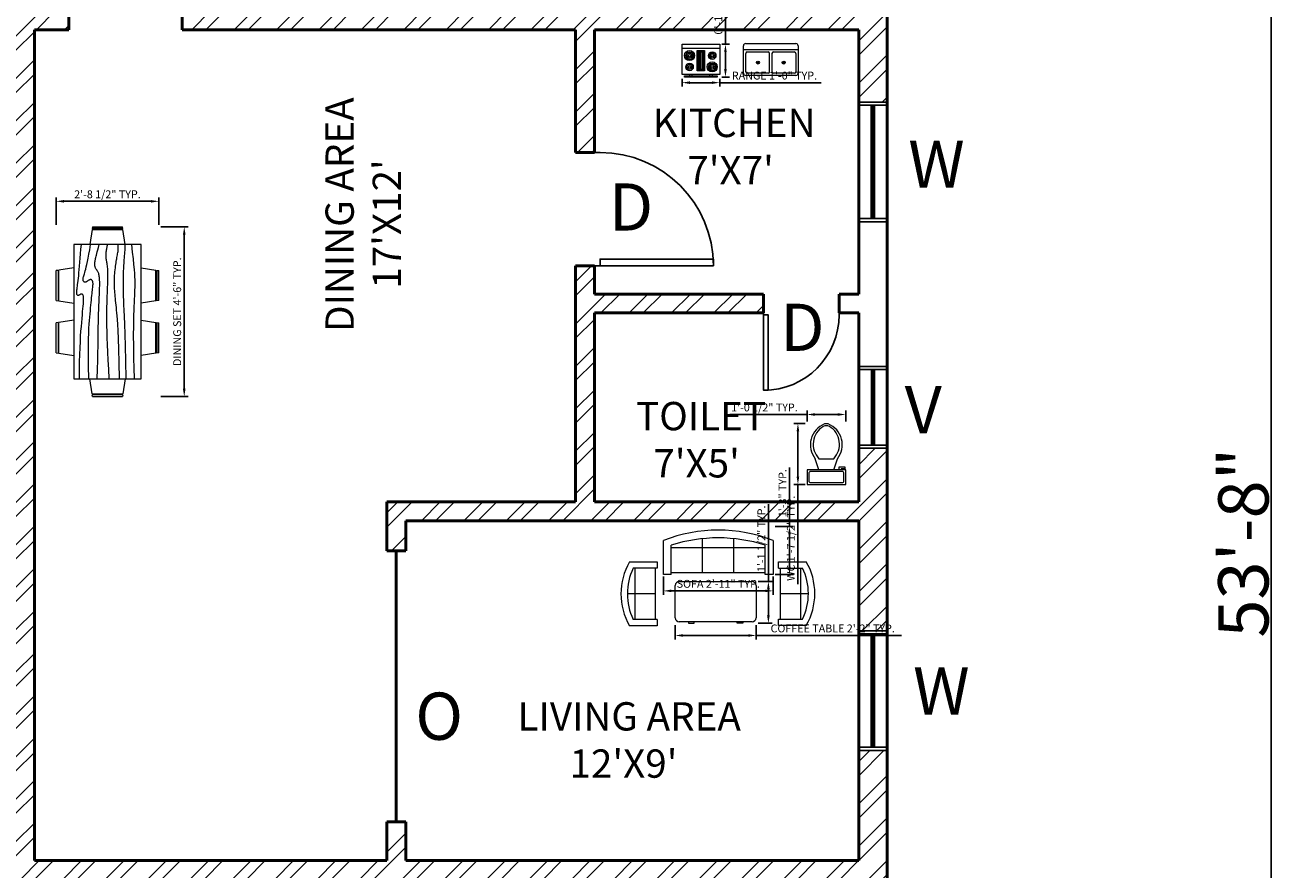
# Model space of a CAD drawing. Units: inches. Extents: x -31485 to -28799, y 18003 to 19130.
# Tile 5 of 15: x -30936 to -30538, y 18398 to 18666. Entities that reach past the tile are written whole.
import ezdxf

# ---------------------------------------------------------------- set-up
doc = ezdxf.new("R2010")
doc.units = ezdxf.units.IN
for name, color, linetype, lineweight in [('A-ANNO-DIMS', 2, 'Continuous', 18), ('A-ANNO-TEXT', 7, 'Continuous', 18), ('A-AREA-IDEN', 7, 'Continuous', 18), ('A-DOOR', 3, 'Continuous', 25), ('A-FLOR-FIXT', 9, 'Continuous', 18), ('A-FURN', 8, 'Continuous', 18), ('A-GLAZ', 4, 'Continuous', 25), ('A-WALL', 7, 'Continuous', 50), ('A-WALL-PATT', 8, 'Continuous', 13)]:
    doc.layers.add(name, color=color, linetype=linetype, lineweight=lineweight)
doc.styles.get("Standard").update_dxf_attribs({"font": 'arial.ttf'})
doc.dimstyles.new('ISO-25', dxfattribs={"dimtxt": 2.5, "dimasz": 2.5, "dimexe": 1.25, "dimexo": 0.625, "dimtad": 1, "dimdec": 0, "dimlunit": 3, "dimtxsty": 'Standard', "dimcen": 2.5, "dimadec": 0, "dimazin": 0, "dimtfac": 1, "dimtdec": 0, "dimtmove": 0, "dimatfit": 3, "dimfxl": 1, "dimarcsym": 0})

# ---------------------------------------------------------------- blocks, each defined once
blk = doc.blocks.new('*U8')
for p, q in [((0, 0), (0, -100)), ((750, 0), (750, -100))]:
    blk.add_line(p, q)
blk.add_lwpolyline([(0, 0), (0, 750), (43.75, 750), (43.75, 0)], close=True)
blk.add_arc((0, 0), 750, 0, 90)
blk = doc.blocks.new('Desk - 30 x 60 in.')
for p, q in [((-26.999995, 0), (26.999995, 0)), ((-29.999995, -27), (-29.999995, -3)), ((29.999995, -3), (29.999995, -27)), ((26.999995, -30), (-26.999995, -30)), ((-20.000005, -30), (-20.000005, -31)), ((-20.000005, -31), (-16.000005, -31)), ((-16.000005, -31), (-16.000005, -30)), ((15.999995, -31), (15.999995, -30)), ((19.999995, -31), (15.999995, -31)), ((19.999995, -30), (19.999995, -31))]:
    blk.add_line(p, q)
for centre, start, end in [((-26.499995, -3.5), 98.1301, 171.8699), ((26.499995, -3.5), 8.130102, 81.8699), ((-26.499995, -26.5), 188.1301, 261.8699), ((26.499995, -26.5), 278.1301, 351.8699)]:
    blk.add_arc(centre, 3.535534, start, end)
blk = doc.blocks.new('Sofa - Roundback 7 ft.')
for p, q in [((-12.00002, -32.4421), (-12.00003, -6.5971)), ((11.99997, -32.4421), (11.99998, -6.5971)), ((-36.000027, -34), (-36.000027, -11.4696)), ((-35.999844, -13.3819), (35.9998, -13.3819)), ((35.99998, -34), (35.99998, -11.4696)), ((-36.000027, -32.4421), (35.99998, -32.4421))]:
    blk.add_line(p, q)
for points in [[(-36.000027, -34), (-42.000027, -34), (-42.000027, -8)], [(41.99998, -8), (41.99998, -34), (35.99998, -34)]]:
    blk.add_lwpolyline(points)
for centre, radius, start, end in [((0, -114.25), 114.25, 68.43141, 111.5686), ((-0.00001, -127.1968), 121.1968, 72.72033, 107.2797)]:
    blk.add_arc(centre, radius, start, end)
blk = doc.blocks.new('Sofa - Roundback Loveseat 5 ft.')
for p, q in [((-24, -33.99998), (-24, -11.46958)), ((0, -32.44198), (0, -5.99998)), ((24.00004, -33.99998), (24.00004, -11.46958)), ((-23.9998, -13.38178), (23.99986, -13.38178)), ((-24, -32.44198), (24.00004, -32.44198))]:
    blk.add_line(p, q)
for points in [[(-24, -33.99998), (-30, -33.99998), (-30, -7.99998)], [(30.00004, -7.99998), (30.00004, -33.99998), (24.00004, -33.99998)]]:
    blk.add_lwpolyline(points)
for centre, radius, start, end in [((0, -60.24998), 60.24998, 60.13715, 119.8628), ((0, -61.38438), 55.38444, 64.32083, 115.6792)]:
    blk.add_arc(centre, radius, start, end)
blk = doc.blocks.new('Dining Set - 36 x 72 in.')
for p, q in [((-22, 27.5), (-22.1562, 26.50042)), ((-22, 27.5), (-6, 27.5)), ((-5.8437, 26.49966), (-6, 27.5)), ((6, 27.5), (5.8438, 26.50042)), ((6, 27.5), (22, 27.5)), ((22.1563, 26.49966), (22, 27.5)), ((-22.2343, 26.00059), (-23.4847, 17.99762)), ((-22.2304, 26), (-5.7608, 26)), ((-5.8416, 26.5), (-22.1534, 26.5)), ((-4.5152, 17.99762), (-5.7655, 25.99926)), ((5.7657, 26.00059), (4.5153, 17.99762)), ((5.7696, 26), (22.2392, 26)), ((22.1584, 26.5), (5.8466, 26.5)), ((23.4848, 17.99762), (22.2345, 25.99926)), ((36, 18), (-36, 18)), ((-36, 18), (-36, -18)), ((36, -18), (36, 18)), ((-45.5, 8), (-44.5004, 8.15617)), ((-45.5, 8), (-45.5, -8)), ((-44.5, -8.15843), (-44.5, 8.15338)), ((-44.0006, 8.23428), (-35.9976, 9.48474)), ((-44, 8.23041), (-44, -8.23915)), ((44.0006, 8.23428), (35.9976, 9.48474)), ((44, 8.23041), (44, -8.23915)), ((44.5, -8.15843), (44.5, 8.15338)), ((45.5, 8), (44.5005, 8.15617)), ((45.5, 8), (45.5, -8)), ((-44.4997, -8.15631), (-45.5, -8)), ((-35.9976, -9.48476), (-43.9993, -8.2345)), ((35.9976, -9.48476), (43.9993, -8.2345)), ((44.4997, -8.15631), (45.5, -8)), ((-36, -18), (36, -18)), ((-22.2343, -26.0006), (-23.4847, -17.99762)), ((-4.5152, -17.99762), (-5.7655, -25.99928)), ((5.7657, -26.0006), (4.5153, -17.99762)), ((23.4848, -17.99762), (22.2345, -25.99928)), ((-22.2304, -26), (-5.7608, -26)), ((-22, -27.5), (-22.1562, -26.50044)), ((-5.8416, -26.5), (-22.1534, -26.5)), ((-5.8437, -26.49967), (-6, -27.5)), ((5.7696, -26), (22.2392, -26)), ((6, -27.5), (5.8438, -26.50044)), ((22.1584, -26.5), (5.8466, -26.5)), ((22.1563, -26.49967), (22, -27.5)), ((-22, -27.5), (-6, -27.5)), ((6, -27.5), (22, -27.5))]:
    blk.add_line(p, q)
for points in [[(-36, 15), (-31.1772, 14.97754), (-26.8079, 14.91406), (-22.8538, 14.81543), (-19.276, 14.6875), (-16.0362, 14.53613), (-13.0957, 14.36718), (-10.4159, 14.18652), (-7.9583, 14), (-5.6904, 13.81315), (-3.6035, 13.63021), (-1.6954, 13.45508), (0.0365, 13.29166), (1.5945, 13.14388), (2.9811, 13.01562), (4.1988, 12.9108), (5.25, 12.83333), (6.1393, 12.78613), (6.8802, 12.76823), (7.4883, 12.77767), (7.9792, 12.8125), (8.3685, 12.87077), (8.6719, 12.95052), (8.9049, 13.0498), (9.0833, 13.16666), (9.2205, 13.29899), (9.3216, 13.44401), (9.3895, 13.59879), (9.4271, 13.76041), (9.4373, 13.92594), (9.4232, 14.09245), (9.3875, 14.257), (9.3333, 14.41666), (9.2638, 14.56917), (9.1836, 14.71484), (9.0975, 14.85465), (9.0104, 14.98958), (8.9272, 15.1206), (8.8529, 15.2487), (8.7922, 15.37483), (8.75, 15.5), (8.7305, 15.62467), (8.7344, 15.74739), (8.7617, 15.86621), (8.8125, 15.97916), (8.8867, 16.08431), (8.9844, 16.17968), (9.1055, 16.26334), (9.25, 16.33333), (9.4189, 16.38802), (9.6172, 16.42708), (9.8506, 16.45052), (10.125, 16.45833), (10.4463, 16.45052), (10.8203, 16.42708), (11.2529, 16.38802), (11.75, 16.33333), (12.3184, 16.26318), (12.9694, 16.17838), (13.7151, 16.07991), (14.5677, 15.96875), (15.5395, 15.84586), (16.6426, 15.71224), (17.8893, 15.56884), (19.2917, 15.41666), (20.859, 15.25667), (22.5879, 15.08984), (24.4721, 14.91715), (26.5052, 14.73958), (28.6809, 14.5581), (30.9929, 14.3737), (33.4347, 14.18733), (36, 14)], [(-36, 10), (-28.9766, 10.14274), (-23.1725, 10.20442), (-18.4241, 10.19775), (-14.5677, 10.13541), (-11.4399, 10.03011), (-8.877, 9.89453), (-6.7154, 9.74137), (-4.7917, 9.58333), (-2.9698, 9.43082), (-1.2246, 9.28515), (0.4415, 9.14534), (2.026, 9.01041), (3.5266, 8.87939), (4.9408, 8.7513), (6.266, 8.62516), (7.5, 8.5), (8.6411, 8.37549), (9.6914, 8.2539), (10.6538, 8.13818), (11.5312, 8.03125), (12.3267, 7.93603), (13.043, 7.85547), (13.6831, 7.79248), (14.25, 7.75), (14.7471, 7.7303), (15.1797, 7.73307), (15.5537, 7.75732), (15.875, 7.80208), (16.1494, 7.86637), (16.3828, 7.94922), (16.5811, 8.04964), (16.75, 8.16666), (16.8944, 8.29915), (17.0143, 8.44531), (17.1089, 8.60319), (17.1771, 8.77083), (17.218, 8.94629), (17.2305, 9.1276), (17.2137, 9.31282), (17.1667, 9.5), (17.0895, 9.6875), (16.987, 9.875), (16.8649, 10.0625), (16.7292, 10.25), (16.5856, 10.4375), (16.4401, 10.625), (16.2985, 10.8125), (16.1667, 11), (16.05, 11.18733), (15.9518, 11.3737), (15.8752, 11.5581), (15.8229, 11.73958), (15.798, 11.91715), (15.8034, 12.08984), (15.842, 12.25667), (15.9167, 12.41666), (16.0295, 12.56836), (16.1784, 12.70833), (16.3605, 12.83268), (16.5729, 12.9375), (16.8127, 13.01888), (17.0768, 13.07291), (17.3625, 13.0957), (17.6667, 13.08333), (17.9894, 13.03312), (18.3418, 12.94726), (18.7382, 12.82918), (19.1927, 12.68229), (19.7195, 12.51001), (20.3327, 12.31575), (21.0465, 12.10294), (21.875, 11.875), (22.8357, 11.63354), (23.959, 11.37304), (25.2786, 11.08618), (26.8282, 10.76562), (28.6414, 10.40405), (30.752, 9.99414), (33.1936, 9.52856), (36, 9)], [(-36, 5.5), (-30.7157, 5.3348), (-26.069, 5.20963), (-21.9946, 5.11767), (-18.4271, 5.05208), (-15.3009, 5.00602), (-12.5508, 4.97265), (-10.1112, 4.94515), (-7.9167, 4.91666), (-5.909, 4.88167), (-4.0586, 4.83984), (-2.3429, 4.79215), (-0.7396, 4.73958), (0.7739, 4.6831), (2.22, 4.6237), (3.6213, 4.56233), (5, 4.5), (6.373, 4.43782), (7.7344, 4.3776), (9.0723, 4.32129), (10.375, 4.27083), (11.6309, 4.22819), (12.8281, 4.19531), (13.9551, 4.17415), (15, 4.16666), (15.954, 4.17448), (16.819, 4.19791), (17.6001, 4.23698), (18.3021, 4.29166), (18.9299, 4.36198), (19.4883, 4.44791), (19.9823, 4.54948), (20.4167, 4.66666), (20.7969, 4.79899), (21.1302, 4.94401), (21.4245, 5.09879), (21.6875, 5.26041), (21.9271, 5.42594), (22.1511, 5.59245), (22.3672, 5.757), (22.5834, 5.91666), (22.8065, 6.06868), (23.0404, 6.21093), (23.2879, 6.34147), (23.5521, 6.45833), (23.8358, 6.55957), (24.142, 6.64323), (24.4735, 6.70735), (24.8334, 6.75), (25.2235, 6.76969), (25.642, 6.76692), (26.0858, 6.74267), (26.5521, 6.69791), (27.0379, 6.63362), (27.5404, 6.55078), (28.0565, 6.45036), (28.5834, 6.33333), (29.1242, 6.19987), (29.7071, 6.04687), (30.3661, 5.87044), (31.1354, 5.66666), (32.0493, 5.43164), (33.142, 5.16146), (34.4475, 4.85221), (36, 4.5)], [(-36, -1), (-30.7915, -0.6591), (-26.0195, -0.38216), (-21.6519, -0.16284), (-17.6563, 0.00521), (-14.0005, 0.12833), (-10.6523, 0.21289), (-7.5796, 0.26522), (-4.75, 0.29166), (-2.134, 0.29793), (0.2878, 0.28711), (2.5317, 0.26163), (4.6146, 0.22396), (6.5529, 0.17651), (8.3633, 0.12174), (10.0623, 0.06209), (11.6667, 0), (13.1899, -0.06201), (14.6341, -0.1211), (15.9982, -0.17432), (17.2813, -0.21875), (18.4823, -0.25147), (19.6003, -0.26953), (20.6343, -0.27002), (21.5834, -0.25), (22.4481, -0.20768), (23.2357, -0.14584), (23.9549, -0.06836), (24.6146, 0.02083), (25.2235, 0.11784), (25.7904, 0.21875), (26.3241, 0.31966), (26.8334, 0.41666), (27.3265, 0.50618), (27.8099, 0.58593), (28.2894, 0.65397), (28.7709, 0.70833), (29.2601, 0.74707), (29.763, 0.76823), (30.2855, 0.76985), (30.8334, 0.75), (31.4088, 0.70784), (31.9994, 0.64713), (32.589, 0.57275), (33.1615, 0.48958), (33.7008, 0.4025), (34.1908, 0.3164), (34.6153, 0.23616), (34.9584, 0.16666), (35.2099, 0.11165), (35.3848, 0.07031), (35.504, 0.04069), (35.5886, 0.02083), (35.6594, 0.00879), (35.7377, 0.0026), (35.8442, 0.00032), (36, 0)], [(-36, -6.5), (-27.1843, -6.31267), (-20.084, -6.1263), (-14.469, -5.9419), (-10.1094, -5.76042), (-6.7752, -5.58285), (-4.2363, -5.41016), (-2.2629, -5.24333), (-0.625, -5.08334), (0.8708, -4.93099), (2.2715, -4.78646), (3.5872, -4.64974), (4.8281, -4.52084), (6.0046, -4.39974), (7.127, -4.28646), (8.2053, -4.18099), (9.25, -4.08334), (10.2705, -3.99382), (11.2734, -3.91407), (12.2647, -3.84603), (13.25, -3.79167), (14.2354, -3.75293), (15.2266, -3.73177), (16.2295, -3.73015), (17.25, -3.75), (18.2912, -3.79248), (19.3451, -3.85547), (20.4009, -3.93604), (21.4479, -4.03125), (22.4754, -4.13819), (23.4727, -4.25391), (24.4289, -4.37549), (25.3334, -4.5), (26.1785, -4.62492), (26.9694, -4.74935), (27.7145, -4.87281), (28.4219, -4.99479), (29.1, -5.11483), (29.7572, -5.23242), (30.4016, -5.34709), (31.0417, -5.45834), (31.6837, -5.56437), (32.3262, -5.65821), (32.9658, -5.73153), (33.599, -5.77604), (34.2224, -5.78345), (34.8327, -5.74545), (35.4264, -5.65373), (36, -5.5)], [(-36, -10), (-26.4022, -9.81299), (-18.4675, -9.62891), (-11.9839, -9.45069), (-6.7396, -9.28125), (-2.5226, -9.12354), (0.8789, -8.98047), (3.6769, -8.85498), (6.0833, -8.75), (8.2767, -8.66765), (10.3021, -8.60677), (12.1712, -8.56543), (13.8958, -8.54167), (15.4876, -8.53353), (16.9583, -8.53907), (18.3197, -8.55632), (19.5834, -8.58334), (20.7616, -8.61841), (21.8685, -8.66081), (22.9188, -8.71004), (23.9271, -8.76563), (24.9081, -8.82707), (25.8763, -8.89388), (26.8465, -8.96558), (27.8334, -9.04167), (28.8474, -9.12118), (29.8828, -9.20117), (30.93, -9.27824), (31.9792, -9.34896), (33.0205, -9.40991), (34.0443, -9.45768), (35.0407, -9.48885), (36, -9.5)], [(-36, -14.5), (-30.0881, -14.33513), (-25.0332, -14.21224), (-20.7312, -14.12647), (-17.0781, -14.07292), (-13.97, -14.04671), (-11.3027, -14.04297), (-8.9724, -14.05681), (-6.875, -14.08334), (-4.9224, -14.11833), (-3.0905, -14.16016), (-1.3709, -14.20785), (0.2448, -14.26042), (1.7647, -14.3169), (3.1973, -14.3763), (4.5507, -14.43767), (5.8333, -14.5), (7.0554, -14.5621), (8.235, -14.62175), (9.3922, -14.67652), (10.5469, -14.72396), (11.7192, -14.76164), (12.929, -14.78711), (14.1965, -14.79794), (15.5417, -14.79167), (16.9933, -14.76424), (18.6152, -14.70508), (20.4804, -14.60197), (22.6615, -14.44271), (25.2312, -14.21509), (28.2624, -13.9069), (31.8277, -13.50594), (36, -13)]]:
    blk.add_lwpolyline(points)
blk = doc.blocks.new('Range-Oven - 30 in top')
for p, q in [((0, -3), (30, -3)), ((12, -6), (18, -6)), ((13, -20), (13, -6)), ((14, -6), (14, -20)), ((15, -20), (15, -6)), ((16, -6), (16, -20)), ((17, -20), (17, -6)), ((6, -24), (6, -25)), ((8, -25), (8, -24)), ((18, -20), (12, -20)), ((22, -25), (22, -24)), ((24, -24), (24, -25))]:
    blk.add_line(p, q)
for points in [[(0, -24), (0, 0), (30, 0), (30, -24)], [(12, -21), (12, -5), (18, -5), (18, -21)], [(2, -26), (2, -25), (28, -25), (28, -26)]]:
    blk.add_lwpolyline(points, close=True)
for centre, radius in [((6, -9), 4), ((6, -9), 3), ((6, -9), 2), ((6, -9), 1), ((24, -9), 3), ((24, -9), 2), ((24, -9), 1), ((6, -18), 3), ((6, -18), 2), ((6, -18), 1), ((24, -18), 4), ((24, -18), 3), ((24, -18), 2), ((24, -18), 1)]:
    blk.add_circle(centre, radius)
blk = doc.blocks.new('Sink-double - 36 in top')
for p, q in [((-18, -4), (18, -4)), ((-0.75, -18.5), (-0.75, -6.5)), ((0.75, -6.5), (0.75, -18.5))]:
    blk.add_line(p, q)
for points in [[(-16.5, 0), (16.5, 0)], [(-18, -19.5), (-18, -1.5)], [(-16.5, -18.5), (-16.5, -6.5)], [(-15.5, -5.5), (-1.75, -5.5)], [(1.75, -5.5), (15.5, -5.5)], [(16.5, -6.5), (16.5, -18.5)], [(18, -1.5), (18, -19.5)], [(16.5, -21), (-16.5, -21)], [(-1.75, -19.5), (-15.5, -19.5)], [(15.5, -19.5), (1.75, -19.5)]]:
    blk.add_lwpolyline(points)
for centre, radius in [((-8.5, -12.5), 1), ((-8.5, -12.5), 0.5), ((8.5, -12.5), 1), ((8.5, -12.5), 0.5)]:
    blk.add_circle(centre, radius)
for centre, radius, start, end in [((-16.5, -1.5), 1.5, 90, 180), ((16.5, -1.5), 1.5, 0, 90), ((-15.5, -6.5), 1, 90, 180), ((-1.75, -6.5), 1, 0, 90), ((1.75, -6.5), 1, 90, 180), ((15.5, -6.5), 1, 0, 90), ((-16.5, -19.5), 1.5, 180, 270), ((-15.5, -18.5), 1, 180, 270), ((-1.75, -18.5), 1, 270, 0), ((1.75, -18.5), 1, 180, 270), ((15.5, -18.5), 1, 270, 0), ((16.5, -19.5), 1.5, 270, 0)]:
    blk.add_arc(centre, radius, start, end)
blk = doc.blocks.new('Toilet - top')
for p, q in [((9.5, -6), (9.5, -2)), ((-10, -8.5), (-8, -8.5)), ((-10, -9.5), (-10, -8.5)), ((-7, -9.5), (-10, -9.5)), ((-8, -8.5), (-8, -8)), ((-7, -8), (-7, -9.5)), ((-4, -8), (-6, -14)), ((4, -8), (6, -14)), ((4, -14), (-4, -14))]:
    blk.add_line(p, q)
blk.add_lwpolyline([(10.5, -8), (10.5, 0), (-10.5, 0), (-10.5, -8)], close=True)
for points in [[(-9.5, -2), (-9.5, -6)], [(8.5, -1), (-8.5, -1)], [(-8.5, -7), (8.5, -7)]]:
    blk.add_lwpolyline(points)
for centre, radius, start, end in [((-8.62, -1.88), 0.884, 81.8699, 188.1301), ((-8.62, -6.12), 0.884, 171.8699, 278.1301), ((8.62, -1.88), 0.884, 351.8699, 98.1301), ((8.62, -6.12), 0.884, 261.8699, 8.1301), ((3.52, -21.58), 12.17, 141.46911, 247.97143), ((4.2, -21.82), 11.33, 136.36773, 238.94682), ((-3.52, -21.58), 12.17, 292.02843, 38.53071), ((-4.2, -21.82), 11.33, 301.05301, 43.63209), ((0, -27.88), 4, 245.73182, 294.26817), ((0, -29), 4, 254.86053, 285.13947)]:
    blk.add_arc(centre, radius, start, end)
blk = doc.blocks.new('*D199')
at = {"layer": 'A-ANNO-DIMS', "color": 0, "lineweight": -2, "transparency": 16777216}
for p, q in [((-30660.9, 18823.8), (-30538.22, 18823.8)), ((-30539.47, 18821.3), (-30539.47, 18182.3)), ((-30660.9, 18179.8), (-30538.22, 18179.8))]:
    blk.add_line(p, q, dxfattribs=at)
at = {"layer": 'A-ANNO-DIMS', "color": 0, "transparency": 16777216}
for points in [[(-30539.88, 18821.3), (-30539.05, 18821.3), (-30539.47, 18823.8)], [(-30539.88, 18182.3), (-30539.05, 18182.3), (-30539.47, 18179.8)]]:
    blk.add_solid(points, dxfattribs=at)
at = {"layer": 'Defpoints', "color": 0, "transparency": 16777216}
for p in [(-30661.53, 18823.8), (-30661.53, 18179.8), (-30539.47, 18179.8)]:
    blk.add_point(p, dxfattribs=at)
at = {"layer": 'A-ANNO-DIMS', "color": 0, "transparency": 16777216, "insert": (-30548.27, 18501.8), "char_height": 2.5, "attachment_point": 5, "rotation": 90}
blk.add_mtext('{\\H6.4x;53\'-8"}', dxfattribs=at)
blk = doc.blocks.new('WIN-900-W9')
for p, q in [((-29982.21, 18824.12), (-29982.21, 18815.12)), ((-29981.21, 18824.12), (-29981.21, 18815.12)), ((-29945.21, 18824.12), (-29945.21, 18815.12)), ((-29944.21, 18824.12), (-29944.21, 18815.12)), ((-29981.21, 18820.12), (-29945.21, 18820.12)), ((-29981.21, 18819.62), (-29945.21, 18819.62)), ((-29981.21, 18819.12), (-29945.21, 18819.12))]:
    blk.add_line(p, q)
blk = doc.blocks.new('VENT-600-W9')
for p, q in [((-29896.21, 18594.12), (-29905.21, 18594.12)), ((-29896.21, 18593.12), (-29905.21, 18593.12)), ((-29901.21, 18593.12), (-29901.21, 18569.12)), ((-29900.71, 18593.12), (-29900.71, 18569.12)), ((-29900.21, 18593.12), (-29900.21, 18569.12)), ((-29896.21, 18569.12), (-29905.21, 18569.12)), ((-29896.21, 18568.12), (-29905.21, 18568.12))]:
    blk.add_line(p, q)
blk = doc.blocks.new('*D232')
at = {"layer": 'A-ANNO-DIMS', "color": 0, "lineweight": -2, "transparency": 16777216}
for p, q in [((-30732.59, 18491.09), (-30732.59, 18485.24)), ((-30697.75, 18491.09), (-30697.75, 18485.24)), ((-30730.09, 18486.49), (-30700.25, 18486.49))]:
    blk.add_line(p, q, dxfattribs=at)
at = {"layer": 'A-ANNO-DIMS', "color": 0, "transparency": 16777216}
for points in [[(-30730.09, 18486.91), (-30730.09, 18486.08), (-30732.59, 18486.49)], [(-30700.25, 18486.91), (-30700.25, 18486.08), (-30697.75, 18486.49)]]:
    blk.add_solid(points, dxfattribs=at)
at = {"layer": 'Defpoints', "color": 0, "transparency": 16777216}
for p in [(-30732.59, 18491.72), (-30697.75, 18491.72), (-30697.75, 18486.49)]:
    blk.add_point(p, dxfattribs=at)
at = {"layer": 'A-ANNO-DIMS', "color": 0, "transparency": 16777216, "insert": (-30715.17, 18488.41), "char_height": 2.5, "attachment_point": 5}
blk.add_mtext('SOFA 2\'-11" TYP.', dxfattribs=at)
blk = doc.blocks.new('*D233')
at = {"layer": 'A-ANNO-DIMS', "color": 0, "lineweight": -2, "transparency": 16777216}
for p, q in [((-30692.53, 18506.93), (-30692.53, 18525.68)), ((-30697.13, 18506.93), (-30691.28, 18506.93)), ((-30692.53, 18494.22), (-30692.53, 18504.43)), ((-30697.13, 18491.72), (-30691.28, 18491.72))]:
    blk.add_line(p, q, dxfattribs=at)
at = {"layer": 'A-ANNO-DIMS', "color": 0, "transparency": 16777216}
for points in [[(-30692.95, 18504.43), (-30692.11, 18504.43), (-30692.53, 18506.93)], [(-30692.95, 18494.22), (-30692.11, 18494.22), (-30692.53, 18491.72)]]:
    blk.add_solid(points, dxfattribs=at)
at = {"layer": 'Defpoints', "color": 0, "transparency": 16777216}
for p in [(-30697.75, 18506.93), (-30692.53, 18506.93), (-30697.75, 18491.72)]:
    blk.add_point(p, dxfattribs=at)
at = {"layer": 'A-ANNO-DIMS', "color": 0, "transparency": 16777216, "insert": (-30694.43, 18517.55), "char_height": 2.5, "attachment_point": 5, "rotation": 90}
blk.add_mtext('1\'-3" TYP.', dxfattribs=at)
blk = doc.blocks.new('*D236')
at = {"layer": 'A-ANNO-DIMS', "color": 0, "lineweight": -2, "transparency": 16777216}
for p, q in [((-30687.59, 18539.64), (-30691.11, 18539.64)), ((-30689.86, 18537.14), (-30689.86, 18522.81)), ((-30687.59, 18520.31), (-30691.11, 18520.31)), ((-30689.86, 18520.31), (-30689.86, 18488.61))]:
    blk.add_line(p, q, dxfattribs=at)
at = {"layer": 'A-ANNO-DIMS', "color": 0, "transparency": 16777216}
for points in [[(-30690.28, 18537.14), (-30689.44, 18537.14), (-30689.86, 18539.64)], [(-30690.28, 18522.81), (-30689.44, 18522.81), (-30689.86, 18520.31)]]:
    blk.add_solid(points, dxfattribs=at)
at = {"layer": 'Defpoints', "color": 0, "transparency": 16777216}
for p in [(-30686.96, 18539.64), (-30689.86, 18520.31), (-30686.96, 18520.31)]:
    blk.add_point(p, dxfattribs=at)
at = {"layer": 'A-ANNO-DIMS', "color": 0, "transparency": 16777216, "insert": (-30691.78, 18503.21), "char_height": 2.5, "attachment_point": 5, "rotation": 90}
blk.add_mtext('WC 1\'-7 1/2" TYP.', dxfattribs=at)
blk = doc.blocks.new('*D237')
at = {"layer": 'A-ANNO-DIMS', "color": 0, "lineweight": -2, "transparency": 16777216}
for p, q in [((-30686.96, 18542.54), (-30711.54, 18542.54)), ((-30686.96, 18540.27), (-30686.96, 18543.79)), ((-30677.18, 18542.54), (-30684.46, 18542.54)), ((-30674.68, 18540.27), (-30674.68, 18543.79))]:
    blk.add_line(p, q, dxfattribs=at)
at = {"layer": 'A-ANNO-DIMS', "color": 0, "transparency": 16777216}
for points in [[(-30684.46, 18542.96), (-30684.46, 18542.13), (-30686.96, 18542.54)], [(-30677.18, 18542.96), (-30677.18, 18542.13), (-30674.68, 18542.54)]]:
    blk.add_solid(points, dxfattribs=at)
at = {"layer": 'Defpoints', "color": 0, "transparency": 16777216}
for p in [(-30686.96, 18542.54), (-30686.96, 18539.64), (-30674.68, 18539.64)]:
    blk.add_point(p, dxfattribs=at)
at = {"layer": 'A-ANNO-DIMS', "color": 0, "transparency": 16777216, "insert": (-30700.5, 18544.46), "char_height": 2.5, "attachment_point": 5}
blk.add_mtext('1\'-0 1/2" TYP.', dxfattribs=at)
blk = doc.blocks.new('*D242')
at = {"layer": 'A-ANNO-DIMS', "color": 0, "lineweight": -2, "transparency": 16777216}
for p, q in [((-30728.9, 18475.57), (-30728.9, 18471.07)), ((-30703.11, 18475.57), (-30703.11, 18471.07)), ((-30726.4, 18472.32), (-30705.61, 18472.32)), ((-30703.11, 18472.32), (-30656.98, 18472.32))]:
    blk.add_line(p, q, dxfattribs=at)
at = {"layer": 'A-ANNO-DIMS', "color": 0, "transparency": 16777216}
for points in [[(-30726.4, 18472.74), (-30726.4, 18471.91), (-30728.9, 18472.32)], [(-30705.61, 18472.74), (-30705.61, 18471.91), (-30703.11, 18472.32)]]:
    blk.add_solid(points, dxfattribs=at)
at = {"layer": 'Defpoints', "color": 0, "transparency": 16777216}
for p in [(-30728.9, 18476.19), (-30703.11, 18476.19), (-30703.11, 18472.32)]:
    blk.add_point(p, dxfattribs=at)
at = {"layer": 'A-ANNO-DIMS', "color": 0, "transparency": 16777216, "insert": (-30678.8, 18474.24), "char_height": 2.5, "attachment_point": 5}
blk.add_mtext('COFFEE TABLE 2\'-2" TYP.', dxfattribs=at)
blk = doc.blocks.new('*D243')
at = {"layer": 'A-ANNO-DIMS', "color": 0, "lineweight": -2, "transparency": 16777216}
for p, q in [((-30699.24, 18489.51), (-30699.24, 18514.09)), ((-30702.49, 18489.51), (-30697.99, 18489.51)), ((-30699.24, 18478.69), (-30699.24, 18487.01)), ((-30702.49, 18476.19), (-30697.99, 18476.19))]:
    blk.add_line(p, q, dxfattribs=at)
at = {"layer": 'A-ANNO-DIMS', "color": 0, "transparency": 16777216}
for points in [[(-30699.66, 18487.01), (-30698.83, 18487.01), (-30699.24, 18489.51)], [(-30699.66, 18478.69), (-30698.83, 18478.69), (-30699.24, 18476.19)]]:
    blk.add_solid(points, dxfattribs=at)
at = {"layer": 'Defpoints', "color": 0, "transparency": 16777216}
for p in [(-30703.11, 18489.51), (-30699.24, 18489.51), (-30703.11, 18476.19)]:
    blk.add_point(p, dxfattribs=at)
at = {"layer": 'A-ANNO-DIMS', "color": 0, "transparency": 16777216, "insert": (-30701.16, 18503.05), "char_height": 2.5, "attachment_point": 5, "rotation": 90}
blk.add_mtext('1\'-1 1/2" TYP.', dxfattribs=at)
blk = doc.blocks.new('*D248')
at = {"layer": 'A-ANNO-DIMS', "color": 0, "lineweight": -2, "transparency": 16777216}
for p, q in [((-30726.7, 18649.16), (-30726.7, 18646.73)), ((-30724.2, 18647.98), (-30717.2, 18647.98)), ((-30714.7, 18649.16), (-30714.7, 18646.73)), ((-30714.7, 18647.98), (-30682.45, 18647.98))]:
    blk.add_line(p, q, dxfattribs=at)
at = {"layer": 'A-ANNO-DIMS', "color": 0, "transparency": 16777216}
for points in [[(-30724.2, 18648.4), (-30724.2, 18647.57), (-30726.7, 18647.98)], [(-30717.2, 18648.4), (-30717.2, 18647.57), (-30714.7, 18647.98)]]:
    blk.add_solid(points, dxfattribs=at)
at = {"layer": 'Defpoints', "color": 0, "transparency": 16777216}
for p in [(-30726.7, 18649.78), (-30714.7, 18649.78), (-30714.7, 18647.98)]:
    blk.add_point(p, dxfattribs=at)
at = {"layer": 'A-ANNO-DIMS', "color": 0, "transparency": 16777216, "insert": (-30697.32, 18649.9), "char_height": 2.5, "attachment_point": 5}
blk.add_mtext('RANGE 1\'-0" TYP.', dxfattribs=at)
blk = doc.blocks.new('*D249')
at = {"layer": 'A-ANNO-DIMS', "color": 0, "lineweight": -2, "transparency": 16777216}
for p, q in [((-30712.9, 18660.18), (-30712.9, 18686.94)), ((-30714.07, 18660.18), (-30711.65, 18660.18)), ((-30712.9, 18652.28), (-30712.9, 18657.68)), ((-30714.07, 18649.78), (-30711.65, 18649.78))]:
    blk.add_line(p, q, dxfattribs=at)
at = {"layer": 'A-ANNO-DIMS', "color": 0, "transparency": 16777216}
for points in [[(-30713.31, 18657.68), (-30712.48, 18657.68), (-30712.9, 18660.18)], [(-30713.31, 18652.28), (-30712.48, 18652.28), (-30712.9, 18649.78)]]:
    blk.add_solid(points, dxfattribs=at)
at = {"layer": 'Defpoints', "color": 0, "transparency": 16777216}
for p in [(-30714.7, 18660.18), (-30712.9, 18660.18), (-30714.7, 18649.78)]:
    blk.add_point(p, dxfattribs=at)
at = {"layer": 'A-ANNO-DIMS', "color": 0, "transparency": 16777216, "insert": (-30714.82, 18674.81), "char_height": 2.5, "attachment_point": 5, "rotation": 90}
blk.add_mtext('0\'-10 1/2" TYP.', dxfattribs=at)
blk = doc.blocks.new('*D260')
at = {"layer": 'A-ANNO-DIMS', "color": 0, "lineweight": -2, "transparency": 16777216}
for p, q in [((-30892.39, 18602.18), (-30883.67, 18602.18)), ((-30884.92, 18550.72), (-30884.92, 18599.68)), ((-30892.39, 18548.22), (-30883.67, 18548.22))]:
    blk.add_line(p, q, dxfattribs=at)
at = {"layer": 'A-ANNO-DIMS', "color": 0, "transparency": 16777216}
for points in [[(-30885.33, 18599.68), (-30884.5, 18599.68), (-30884.92, 18602.18)], [(-30885.33, 18550.72), (-30884.5, 18550.72), (-30884.92, 18548.22)]]:
    blk.add_solid(points, dxfattribs=at)
at = {"layer": 'Defpoints', "color": 0, "transparency": 16777216}
for p in [(-30893.01, 18602.18), (-30884.92, 18602.18), (-30893.01, 18548.22)]:
    blk.add_point(p, dxfattribs=at)
at = {"layer": 'A-ANNO-DIMS', "color": 0, "transparency": 16777216, "insert": (-30886.83, 18575.2), "char_height": 2.5, "attachment_point": 5, "rotation": 90}
blk.add_mtext('DINING SET 4\'-6" TYP.', dxfattribs=at)
blk = doc.blocks.new('*D261')
at = {"layer": 'A-ANNO-DIMS', "color": 0, "lineweight": -2, "transparency": 16777216}
for p, q in [((-30925.63, 18602.81), (-30925.63, 18611.53)), ((-30895.51, 18610.28), (-30923.13, 18610.28)), ((-30893.01, 18602.81), (-30893.01, 18611.53))]:
    blk.add_line(p, q, dxfattribs=at)
at = {"layer": 'A-ANNO-DIMS', "color": 0, "transparency": 16777216}
for points in [[(-30923.13, 18610.69), (-30923.13, 18609.86), (-30925.63, 18610.28)], [(-30895.51, 18610.69), (-30895.51, 18609.86), (-30893.01, 18610.28)]]:
    blk.add_solid(points, dxfattribs=at)
at = {"layer": 'Defpoints', "color": 0, "transparency": 16777216}
for p in [(-30925.63, 18610.28), (-30925.63, 18602.18), (-30893.01, 18602.18)]:
    blk.add_point(p, dxfattribs=at)
at = {"layer": 'A-ANNO-DIMS', "color": 0, "transparency": 16777216, "insert": (-30909.32, 18612.19), "char_height": 2.5, "attachment_point": 5}
blk.add_mtext('2\'-8 1/2" TYP.', dxfattribs=at)

msp = doc.modelspace()

# ---------------------------------------------------------------- hatches: boundary and pattern name
at = {"layer": 'A-WALL-PATT'}
h = msp.add_hatch(dxfattribs=at)
h.set_pattern_fill('ANSI32', color=256)
h.set_pattern_definition([(45, (-1687.357, -0.313), (-6.735192, 6.735192), []), (45, (-1682.867, -0.313), (-6.735192, 6.735192), [])])
h.paths.add_polyline_path([(-31156.53, 18823.8), (-31209.53, 18823.8), (-31209.53, 18761.8), (-31200.53, 18761.8), (-31200.53, 18814.8), (-31156.53, 18814.8)], flags=17)
h.paths.add_polyline_path([(-31022.53, 18823.8), (-31118.53, 18823.8), (-31118.53, 18814.8), (-31074.53, 18814.8), (-31074.53, 18720.79), (-31070.96, 18720.79), (-31068.53, 18720.76), (-31068.53, 18814.8), (-31022.53, 18814.8)], flags=17)
h.paths.add_polyline_path([(-30754.53, 18823.8), (-30850.53, 18823.8), (-30850.53, 18814.8), (-30806.53, 18814.8), (-30806.53, 18723.1), (-30800.53, 18723.1), (-30800.53, 18814.8), (-30754.53, 18814.8)], flags=17)
h.paths.add_polyline_path([(-30661.53, 18823.8), (-30716.53, 18823.8), (-30716.53, 18814.8), (-30670.53, 18814.8), (-30670.53, 18761.8), (-30661.53, 18761.8)], flags=17)
h.paths.add_polyline_path([(-30986.92, 18670.8), (-31068.53, 18670.8), (-31068.53, 18684.76), (-31074.53, 18684.76), (-31074.53, 18670.8), (-31200.53, 18670.8), (-31200.53, 18723.8), (-31209.53, 18723.8), (-31209.53, 18641.8), (-31200.53, 18641.8), (-31200.53, 18664.8), (-31104.53, 18664.8), (-31104.53, 18628.93), (-31098.53, 18628.93), (-31098.53, 18664.8), (-30986.92, 18664.8)], flags=17)
h.paths.add_polyline_path([(-30661.53, 18723.8), (-30670.53, 18723.8), (-30670.53, 18670.8), (-30800.53, 18670.8), (-30800.53, 18687.1), (-30806.53, 18687.1), (-30806.53, 18670.8), (-30885.6, 18670.8), (-30885.6, 18667.8), (-30885.6, 18664.8), (-30760.53, 18664.8), (-30760.53, 18625.8), (-30754.53, 18625.8), (-30754.53, 18664.8), (-30670.53, 18664.8), (-30670.53, 18641.8), (-30661.53, 18641.8)], flags=17)
h.paths.add_polyline_path([(-31200.53, 18574.8), (-31188.56, 18574.8), (-31188.56, 18580.8), (-31200.53, 18580.8), (-31200.53, 18603.8), (-31209.53, 18603.8), (-31209.53, 18557.8), (-31200.53, 18557.8)], flags=17)
h.paths.add_polyline_path([(-31098.53, 18592.93), (-31104.53, 18592.93), (-31104.53, 18580.8), (-31164.56, 18580.8), (-31164.56, 18574.8), (-31104.53, 18574.8), (-31104.53, 18514.8), (-31200.53, 18514.8), (-31200.53, 18531.8), (-31209.53, 18531.8), (-31209.53, 18473.8), (-31200.53, 18473.8), (-31200.53, 18508.8), (-31056.53, 18508.8), (-31056.53, 18501.62), (-31050.53, 18501.62), (-31050.53, 18514.8), (-31098.53, 18514.8)], flags=17)
h.paths.add_polyline_path([(-30661.53, 18531.8), (-30670.53, 18531.8), (-30670.53, 18514.8), (-30754.53, 18514.8), (-30754.53, 18574.8), (-30700.75, 18574.8), (-30700.75, 18577.44), (-30700.75, 18580.8), (-30754.53, 18580.8), (-30754.53, 18589.8), (-30760.53, 18589.8), (-30760.53, 18514.8), (-30820.53, 18514.8), (-30820.53, 18499.26), (-30814.53, 18499.26), (-30814.53, 18508.8), (-30670.53, 18508.8), (-30670.53, 18473.8), (-30661.53, 18473.8)], flags=17)
h.paths.add_polyline_path([(-30661.53, 18435.8), (-30670.53, 18435.8), (-30670.53, 18400.8), (-30814.53, 18400.8), (-30814.53, 18413.15), (-30820.53, 18413.15), (-30820.53, 18400.8), (-30932.53, 18400.8), (-30932.53, 18664.8), (-30921.6, 18664.8), (-30921.6, 18670.8), (-30932.53, 18670.8), (-30932.53, 18814.8), (-30888.53, 18814.8), (-30888.53, 18823.8), (-30984.53, 18823.8), (-30984.53, 18814.8), (-30938.53, 18814.8), (-30938.53, 18670.8), (-30950.92, 18670.8), (-30950.92, 18664.8), (-30938.53, 18664.8), (-30938.53, 18400.8), (-31050.53, 18400.8), (-31050.53, 18411.18), (-31056.53, 18411.18), (-31056.53, 18400.8), (-31200.53, 18400.8), (-31200.53, 18435.8), (-31209.53, 18435.8), (-31209.53, 18179.8), (-31200.53, 18179.8), (-31200.53, 18394.8), (-31001.53, 18394.8), (-31001.53, 18179.8), (-30954.53, 18179.8), (-30954.53, 18188.8), (-30995.53, 18188.8), (-30995.53, 18394.8), (-30875.53, 18394.8), (-30875.53, 18188.8), (-30916.53, 18188.8), (-30916.53, 18179.8), (-30869.53, 18179.8), (-30869.53, 18394.8), (-30670.53, 18394.8), (-30670.53, 18179.8), (-30661.53, 18179.8)])

# ---------------------------------------------------------------- linework, layer by layer
at = {"layer": 'A-WALL'}
for p, q in [((-30661.53, 18823.8), (-30661.53, 18179.8)), ((-30921.6, 18670.8), (-30921.6, 18664.8)), ((-30885.6, 18670.8), (-30885.6, 18664.8)), ((-30932.53, 18664.8), (-30921.6, 18664.8)), ((-30932.53, 18664.8), (-30932.53, 18400.8)), ((-30885.6, 18664.8), (-30760.53, 18664.8)), ((-30760.53, 18664.8), (-30760.53, 18625.8)), ((-30754.53, 18664.8), (-30670.53, 18664.8)), ((-30754.53, 18664.8), (-30754.53, 18625.8)), ((-30670.53, 18664.8), (-30670.53, 18580.8)), ((-30760.53, 18625.8), (-30754.53, 18625.8)), ((-30760.53, 18589.8), (-30760.53, 18514.8)), ((-30760.53, 18589.8), (-30754.53, 18589.8)), ((-30754.53, 18589.8), (-30754.53, 18580.8)), ((-30754.53, 18580.8), (-30700.75, 18580.8)), ((-30700.75, 18580.8), (-30700.75, 18574.8)), ((-30676.75, 18580.8), (-30670.53, 18580.8)), ((-30676.75, 18580.8), (-30676.75, 18574.8)), ((-30754.53, 18574.8), (-30700.75, 18574.8)), ((-30754.53, 18574.8), (-30754.53, 18514.8)), ((-30676.75, 18574.8), (-30670.53, 18574.8)), ((-30670.53, 18574.8), (-30670.53, 18514.8)), ((-30820.53, 18514.8), (-30760.53, 18514.8)), ((-30820.53, 18514.8), (-30820.53, 18499.26)), ((-30754.53, 18514.8), (-30670.53, 18514.8)), ((-30814.53, 18508.8), (-30670.53, 18508.8)), ((-30814.53, 18508.8), (-30814.53, 18499.26)), ((-30670.53, 18508.8), (-30670.53, 18400.8)), ((-30820.53, 18499.26), (-30814.53, 18499.26)), ((-30817.53, 18499.26), (-30817.53, 18413.15)), ((-30820.53, 18413.15), (-30820.53, 18400.8)), ((-30820.53, 18413.15), (-30814.53, 18413.15)), ((-30814.53, 18413.15), (-30814.53, 18400.8)), ((-30932.53, 18400.8), (-30820.53, 18400.8)), ((-30814.53, 18400.8), (-30670.53, 18400.8))]:
    msp.add_line(p, q, dxfattribs=at)

# ---------------------------------------------------------------- block references
at = {"layer": 'A-DOOR'}
for p, xscale, yscale, zscale, rotation in [((-30752.73, 18589.8), -0.0479999995519333, 0.0479999995519333, 0.0479999995519333, 270), ((-30700.75, 18574.24), -0.0320036543541351, 0.0320036543541351, 0.0320036543541351, 180)]:
    msp.add_blockref('*U8', p, dxfattribs=dict(at, xscale=xscale, yscale=yscale, zscale=zscale, rotation=rotation))
at = {"layer": 'A-FLOR-FIXT'}
for name, p, xscale, yscale, zscale in [('Range-Oven - 30 in top', (-30726.7, 18660.18), 0.4, 0.4, 0.4), ('Sink-double - 36 in top', (-30698.48, 18660.4), 0.4823765274114516, 0.4823765274114516, 0.4823765274114516)]:
    msp.add_blockref(name, p, dxfattribs=dict(at, xscale=xscale, yscale=yscale, zscale=zscale))
at = {"layer": 'A-FLOR-FIXT', "xscale": 0.5850068734066302, "yscale": 0.5850068734066302, "zscale": 0.5850068734066302, "rotation": 180}
msp.add_blockref('Toilet - top', (-30680.82, 18520.31), dxfattribs=at)
at = {"layer": 'A-FURN'}
for name, p, xscale, yscale, zscale, rotation in [('Dining Set - 36 x 72 in.', (-30909.32, 18575.2), 0.5930176886900861, 0.5930176886900861, 0.5930176886900861, 90), ('Sofa - Roundback Loveseat 5 ft.', (-30746.1, 18485.55), 0.3381495698466857, 0.3381495698466857, 0.3381495698466857, 89.99999999999999), ('Sofa - Roundback Loveseat 5 ft.', (-30684.49, 18485.63), 0.3381495698466857, 0.3381495698466857, 0.3381495698466857, 270)]:
    msp.add_blockref(name, p, dxfattribs=dict(at, xscale=xscale, yscale=yscale, zscale=zscale, rotation=rotation))
for name, p, xscale, yscale, zscale in [('Sofa - Roundback 7 ft.', (-30715.17, 18505.82), 0.4147575827902149, 0.4147575827902149, 0.4147575827902149), ('Desk - 30 x 60 in.', (-30716, 18489.51), 0.4297812202416646, 0.4297812202416646, 0.4297812202416646)]:
    msp.add_blockref(name, p, dxfattribs=dict(at, xscale=xscale, yscale=yscale, zscale=zscale))
at = {"layer": 'A-GLAZ'}
for name, p, rotation in [('WIN-900-W9', (-11846.41, 48586.01), 89.9999999999743), ('VENT-600-W9', (-60566.73, 37125.92), 180), ('WIN-900-W9', (-11846.41, 48418.01), 89.9999999999743)]:
    msp.add_blockref(name, p, dxfattribs=dict(at, rotation=rotation))

# ---------------------------------------------------------------- texts
at = {"layer": 'A-ANNO-TEXT', "char_height": 15, "attachment_point": 1}
for s, insert in [('{W}', (-30654.8, 18629.57)), ('{D}', (-30749.94, 18615.98)), ('{D}', (-30695.49, 18577.74)), ('{V}', (-30655.91, 18551.58)), ('{W}', (-30653.25, 18462.18)), ('{O}', (-30811.47, 18454.17))]:
    msp.add_mtext_dynamic_manual_height_columns(s, width=638.549, gutter_width=12.5, heights=[0], dxfattribs=dict(at, insert=insert))
at = {"layer": 'A-AREA-IDEN', "insert": (-30840.02, 18568.76), "char_height": 9, "attachment_point": 1, "rotation": 90}
msp.add_mtext_dynamic_manual_height_columns("{DINING AREA\\P     17'X12'}", width=763.1479, gutter_width=12.5, heights=[0], dxfattribs=at)
at = {"layer": 'A-AREA-IDEN', "char_height": 9, "attachment_point": 1}
for s, insert in [("{   KITCHEN\\P       7'X7'}", (-30744.27, 18639.69)), ("{    TOILET\\P      7'X5'}", (-30752.31, 18546.53)), ("{LIVING AREA\\P      12'X9'}", (-30778.96, 18451.12))]:
    msp.add_mtext_dynamic_manual_height_columns(s, width=763.1479, gutter_width=12.5, heights=[0], dxfattribs=dict(at, insert=insert))

# ---------------------------------------------------------------- dimensions: what is measured, and where the dimension line sits
at = {"layer": 'A-ANNO-DIMS'}
for base, p1, p2, angle, text, override, picture, middle in [((-30539.47, 18179.8), (-30661.53, 18823.8), (-30661.53, 18179.8), 90, '{\\H6.4x;<>}', {"dimclrd": 0, "dimclre": 0, "dimclrt": 0}, '*D199', (-30548.27, 18501.8)), ((-30712.9, 18660.18), (-30714.7, 18649.78), (-30714.7, 18660.18), 90, '<> TYP.', {"dimdec": 1, "dimlfac": 1, "dimrnd": 0, "dimzin": 1, "dimdsep": 46, "dimlunit": 4, "dimfrac": 2}, '*D249', (-30714.82, 18674.81)), ((-30925.63, 18610.28), (-30893.01, 18602.18), (-30925.63, 18602.18), 180, '<> TYP.', {"dimdec": 1, "dimlfac": 1, "dimrnd": 0, "dimzin": 1, "dimdsep": 46, "dimlunit": 4, "dimfrac": 2}, '*D261', (-30909.32, 18612.19)), ((-30884.92, 18602.18), (-30893.01, 18548.22), (-30893.01, 18602.18), 90, 'DINING SET <> TYP.', {"dimdec": 1, "dimlfac": 1, "dimrnd": 0, "dimzin": 1, "dimdsep": 46, "dimlunit": 4, "dimfrac": 2}, '*D260', (-30886.83, 18575.2)), ((-30686.96, 18542.54), (-30674.68, 18539.64), (-30686.96, 18539.64), 180, '<> TYP.', {"dimdec": 1, "dimlfac": 1, "dimrnd": 0, "dimzin": 1, "dimdsep": 46, "dimlunit": 4, "dimfrac": 2}, '*D237', (-30700.5, 18544.46)), ((-30689.86, 18520.31), (-30686.96, 18539.64), (-30686.96, 18520.31), 270, 'WC <> TYP.', {"dimdec": 1, "dimlfac": 1, "dimrnd": 0, "dimzin": 1, "dimdsep": 46, "dimlunit": 4, "dimfrac": 2}, '*D236', (-30691.78, 18503.21)), ((-30692.53, 18506.93), (-30697.75, 18491.72), (-30697.75, 18506.93), 90, '<> TYP.', {"dimdec": 1, "dimlfac": 1, "dimrnd": 0, "dimzin": 1, "dimdsep": 46, "dimlunit": 4, "dimfrac": 2}, '*D233', (-30694.43, 18517.55)), ((-30699.24, 18489.51), (-30703.11, 18476.19), (-30703.11, 18489.51), 90, '<> TYP.', {"dimdec": 1, "dimlfac": 1, "dimrnd": 0, "dimzin": 1, "dimdsep": 46, "dimlunit": 4, "dimfrac": 2}, '*D243', (-30701.16, 18503.05))]:
    dim = msp.add_linear_dim(base=base, p1=p1, p2=p2, angle=angle, text=text, dimstyle='ISO-25', override=override, dxfattribs=at)
    dim.commit()
    dim.dimension.update_dxf_attribs({"geometry": picture, "text_midpoint": middle})
for base, p1, p2, text, picture, middle in [((-30714.7, 18647.98), (-30726.7, 18649.78), (-30714.7, 18649.78), 'RANGE <> TYP.', '*D248', (-30697.32, 18649.9)), ((-30697.75, 18486.49), (-30732.59, 18491.72), (-30697.75, 18491.72), 'SOFA <> TYP.', '*D232', (-30715.17, 18488.41)), ((-30703.11, 18472.32), (-30728.9, 18476.19), (-30703.11, 18476.19), 'COFFEE TABLE <> TYP.', '*D242', (-30678.8, 18474.24))]:
    dim = msp.add_linear_dim(base=base, p1=p1, p2=p2, text=text, dimstyle='ISO-25', override={"dimdec": 1, "dimlfac": 1, "dimrnd": 0, "dimzin": 1, "dimdsep": 46, "dimlunit": 4, "dimfrac": 2}, dxfattribs=at)
    dim.commit()
    dim.dimension.update_dxf_attribs({"geometry": picture, "text_midpoint": middle})

doc.saveas('drawing.dxf')
